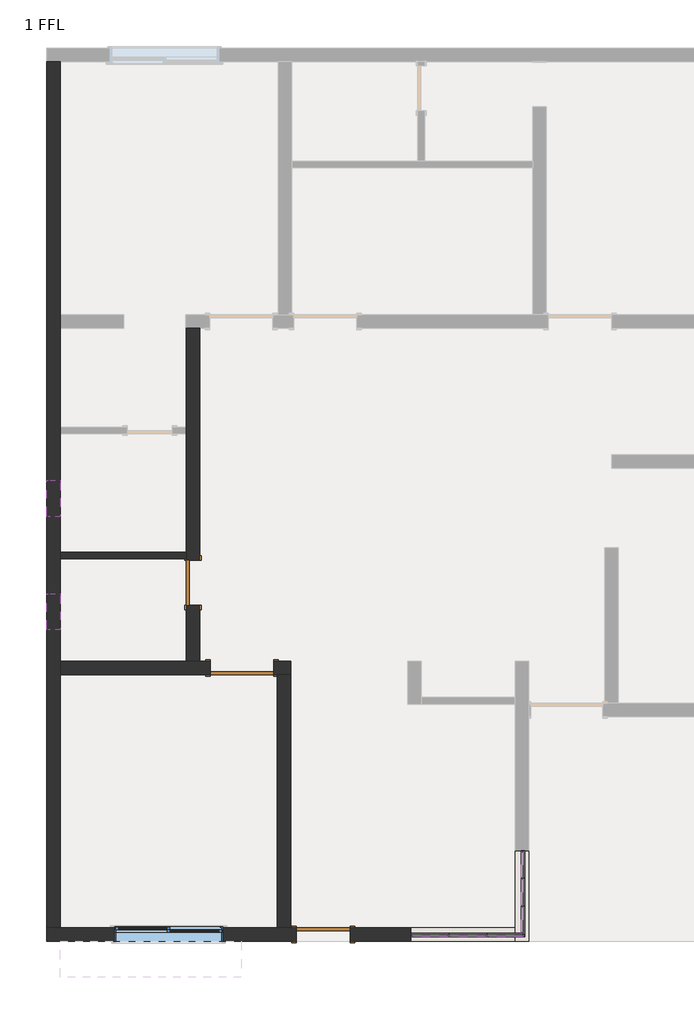
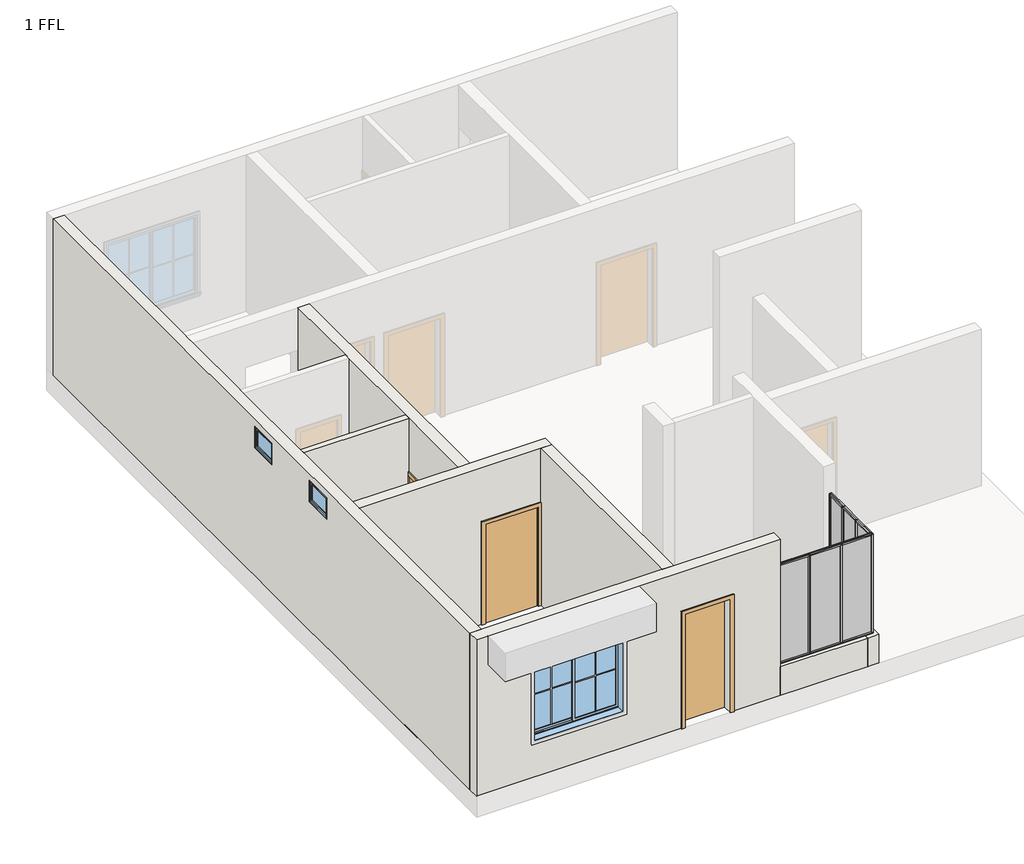
# One storey, part 1 of 2: 23 members, 9 plates, 8 walls, 3 doors, 3 windows.
"""IFC4 building model written with IfcOpenShell, lengths in millimetres."""

from ifc_helpers import new_model, si_unit, origin, origin_with_axes, place, context, project, spatial, polyline, outline, extrude, faceted_brep, transform, mapped, element, save
from components import single_flush_0848dd25, single_flush_bath_bb98abfd, single_flush_md_2_ea82e2eb, member_0e6c94ff, member_b561e846, member_158a8462, member_dd05f1c1, member_cc9ef0d5, member_a5642750, member_968ff67a, member_910a056f, member_3995c9cc, member_c125f493, member_90203b35, system_panel_glazed_d35b251a, system_panel_glazed_6aed1af6, system_panel_glazed_7e3d14c9, fixed_v_1ea75518, window_sliding_double_89c6b595

model = new_model("IFC4")

# Units and contexts
model_context = context("Model", 3, world=origin())
ifc_project = project(units=[si_unit("LENGTHUNIT", "METRE", prefix="MILLI")], contexts=[model_context])

# Site, building, storey
site = spatial("IfcSite", under=ifc_project)
building = spatial("IfcBuilding", under=site)
storey = spatial("IfcBuildingStorey", under=building, Name="1 FFL", Elevation=0.0)

# Doors
placement = place(None, origin())
single_flush_shape = single_flush_0848dd25(model_context)
element("IfcDoor", 1, ObjectType="Single-Flush", at=placement, inside=storey, context=model_context, shape_type="MappedRepresentation", body=[
    mapped(single_flush_shape, transform((-1780.0942549, -3341.3296941, 0.0), x_axis=(1.0, 0.0, 0.0), y_axis=(0.0, 1.0, 0.0), z_axis=(0.0, 0.0, 1.0))),
])
single_flush_bath_shape = single_flush_bath_bb98abfd(model_context)
element("IfcDoor", 2, ObjectType="Single-Flush : BATH", at=placement, inside=storey, context=model_context, shape_type="MappedRepresentation", body=[
    mapped(single_flush_bath_shape, transform((-2605.5942549, -1895.6547785, 0.0), x_axis=(0.0, 1.0, 0.0), y_axis=(-1.0, 0.0, 0.0), z_axis=(0.0, 0.0, 1.0))),
])
single_flush_md_2_shape = single_flush_md_2_ea82e2eb(model_context)
element("IfcDoor", 3, ObjectType="Single-Flush : MD 2", at=placement, inside=storey, context=model_context, shape_type="MappedRepresentation", body=[
    mapped(single_flush_md_2_shape, transform((-408.4942549, -7846.758484, 0.0), x_axis=(-1.0, 0.0, 0.0), y_axis=(0.0, -1.0, 0.0), z_axis=(0.0, 0.0, 1.0))),
])

# Members
member_shape = member_0e6c94ff(model_context)
element("IfcMember", 4, ObjectType="Rectangular Mullion : 1\" Square", at=placement, inside=storey, context=model_context, shape_type="MappedRepresentation", body=[
    mapped(member_shape, transform((2957.0057451, -7811.7296941, 2743.2), x_axis=(0.0, 0.0, 1.0), y_axis=(-1.0, 0.0, 0.0), z_axis=(0.0, -1.0, 0.0))),
])
element("IfcMember", 5, ObjectType="Rectangular Mullion : 1\" Square", at=placement, inside=storey, context=model_context, shape_type="MappedRepresentation", body=[
    mapped(member_shape, transform((2957.0057451, -6884.6296941, 2743.2), x_axis=(0.0, 0.0, 1.0), y_axis=(-1.0, 0.0, 0.0), z_axis=(0.0, -1.0, 0.0))),
])
element("IfcMember", 6, ObjectType="Rectangular Mullion : 1\" Square", at=placement, inside=storey, context=model_context, shape_type="MappedRepresentation", body=[
    mapped(member_shape, transform((2957.0057451, -6452.8296941, 609.6), x_axis=(0.0, 0.0, -1.0), y_axis=(-1.0, 0.0, 0.0), z_axis=(0.0, 1.0, 0.0))),
])
element("IfcMember", 7, ObjectType="Rectangular Mullion : 1\" Square", at=placement, inside=storey, context=model_context, shape_type="MappedRepresentation", body=[
    mapped(member_shape, transform((2957.0057451, -7379.9296941, 609.6), x_axis=(0.0, 0.0, -1.0), y_axis=(-1.0, 0.0, 0.0), z_axis=(0.0, 1.0, 0.0))),
])
member_2_shape = member_b561e846(model_context)
element("IfcMember", 8, ObjectType="Rectangular Mullion : 1\" Square", at=placement, inside=storey, context=model_context, shape_type="MappedRepresentation", body=[
    mapped(member_2_shape, transform((2957.0057451, -7367.2296941, 609.6), x_axis=(0.0, -1.0, 0.0), y_axis=(-1.0, 0.0, 0.0), z_axis=(0.0, 0.0, -1.0))),
])
element("IfcMember", 9, ObjectType="Rectangular Mullion : 1\" Square", at=placement, inside=storey, context=model_context, shape_type="MappedRepresentation", body=[
    mapped(member_2_shape, transform((2957.0057451, -6897.3296941, 609.6), x_axis=(0.0, -1.0, 0.0), y_axis=(-1.0, 0.0, 0.0), z_axis=(0.0, 0.0, -1.0))),
])
member_3_shape = member_158a8462(model_context)
element("IfcMember", 10, ObjectType="Rectangular Mullion : 1\" Square", at=placement, inside=storey, context=model_context, shape_type="MappedRepresentation", body=[
    mapped(member_3_shape, transform((2957.0057451, -6910.0296941, 609.6), x_axis=(0.0, 0.0, -1.0), y_axis=(-1.0, 0.0, 0.0), z_axis=(0.0, 1.0, 0.0))),
])
element("IfcMember", 11, ObjectType="Rectangular Mullion : 1\" Square", at=placement, inside=storey, context=model_context, shape_type="MappedRepresentation", body=[
    mapped(member_3_shape, transform((2957.0057451, -7354.5296941, 2743.2), x_axis=(0.0, 0.0, 1.0), y_axis=(-1.0, 0.0, 0.0), z_axis=(0.0, -1.0, 0.0))),
])
member_4_shape = member_dd05f1c1(model_context)
element("IfcMember", 12, ObjectType="Rectangular Mullion : 1\" Square", at=placement, inside=storey, context=model_context, shape_type="MappedRepresentation", body=[
    mapped(member_4_shape, transform((2957.0057451, -6427.4296941, 2743.2), x_axis=(0.0, 1.0, 0.0), y_axis=(-1.0, 0.0, 0.0), z_axis=(0.0, 0.0, 1.0))),
])
element("IfcMember", 13, ObjectType="Rectangular Mullion : 1\" Square", at=placement, inside=storey, context=model_context, shape_type="MappedRepresentation", body=[
    mapped(member_4_shape, transform((2957.0057451, -7837.1296941, 609.6), x_axis=(0.0, -1.0, 0.0), y_axis=(-1.0, 0.0, 0.0), z_axis=(0.0, 0.0, -1.0))),
])
member_5_shape = member_cc9ef0d5(model_context)
element("IfcMember", 14, ObjectType="Rectangular Mullion : 1\" Square", at=placement, inside=storey, context=model_context, shape_type="MappedRepresentation", body=[
    mapped(member_5_shape, transform((2977.9478614, -7869.7205876, 2743.2), x_axis=(0.0, 0.0, 1.0), y_axis=(0.0, -1.0, 0.0), z_axis=(1.0, 0.0, 0.0))),
])
element("IfcMember", 15, ObjectType="Rectangular Mullion : 1\" Square", at=placement, inside=storey, context=model_context, shape_type="MappedRepresentation", body=[
    mapped(member_5_shape, transform((1703.7145281, -7869.7205876, 2743.2), x_axis=(0.0, 0.0, 1.0), y_axis=(0.0, -1.0, 0.0), z_axis=(1.0, 0.0, 0.0))),
])
member_6_shape = member_a5642750(model_context)
element("IfcMember", 16, ObjectType="Rectangular Mullion : 1\" Square", at=placement, inside=storey, context=model_context, shape_type="MappedRepresentation", body=[
    mapped(member_6_shape, transform((1072.9478614, -7869.7205876, 609.6), x_axis=(0.0, 0.0, -1.0), y_axis=(0.0, -1.0, 0.0), z_axis=(-1.0, 0.0, 0.0))),
])
member_7_shape = member_968ff67a(model_context)
element("IfcMember", 17, ObjectType="Rectangular Mullion : 1\" Square", at=placement, inside=storey, context=model_context, shape_type="MappedRepresentation", body=[
    mapped(member_7_shape, transform((1703.7145281, -7869.7205876, 615.95), x_axis=(0.0, 0.0, 1.0), y_axis=(0.0, -1.0, 0.0), z_axis=(1.0, 0.0, 0.0))),
])
element("IfcMember", 18, ObjectType="Rectangular Mullion : 1\" Square", at=placement, inside=storey, context=model_context, shape_type="MappedRepresentation", body=[
    mapped(member_7_shape, transform((2977.9478614, -7869.7205876, 615.95), x_axis=(0.0, 0.0, 1.0), y_axis=(0.0, -1.0, 0.0), z_axis=(1.0, 0.0, 0.0))),
])
member_8_shape = member_910a056f(model_context)
element("IfcMember", 19, ObjectType="Rectangular Mullion : 1\" Square", at=placement, inside=storey, context=model_context, shape_type="MappedRepresentation", body=[
    mapped(member_8_shape, transform((2347.1811947, -7869.7205876, 615.95), x_axis=(0.0, 0.0, 1.0), y_axis=(0.0, -1.0, 0.0), z_axis=(1.0, 0.0, 0.0))),
])
element("IfcMember", 20, ObjectType="Rectangular Mullion : 1\" Square", at=placement, inside=storey, context=model_context, shape_type="MappedRepresentation", body=[
    mapped(member_6_shape, transform((2359.8811947, -7869.7205876, 609.6), x_axis=(0.0, 0.0, -1.0), y_axis=(0.0, -1.0, 0.0), z_axis=(-1.0, 0.0, 0.0))),
])
element("IfcMember", 21, ObjectType="Rectangular Mullion : 1\" Square", at=placement, inside=storey, context=model_context, shape_type="MappedRepresentation", body=[
    mapped(member_6_shape, transform((1716.4145281, -7869.7205876, 609.6), x_axis=(0.0, 0.0, -1.0), y_axis=(0.0, -1.0, 0.0), z_axis=(-1.0, 0.0, 0.0))),
])
member_9_shape = member_3995c9cc(model_context)
element("IfcMember", 22, ObjectType="Rectangular Mullion : 1\" Square", at=placement, inside=storey, context=model_context, shape_type="MappedRepresentation", body=[
    mapped(member_9_shape, transform((2347.1811947, -7869.7205876, 2743.2), x_axis=(0.0, 0.0, 1.0), y_axis=(0.0, -1.0, 0.0), z_axis=(1.0, 0.0, 0.0))),
])
member_10_shape = member_c125f493(model_context)
element("IfcMember", 23, ObjectType="Rectangular Mullion : 1\" Square", at=placement, inside=storey, context=model_context, shape_type="MappedRepresentation", body=[
    mapped(member_10_shape, transform((2359.8811947, -7869.7205876, 603.25), x_axis=(1.0, 0.0, 0.0), y_axis=(0.0, -1.0, 0.0), z_axis=(0.0, 0.0, -1.0))),
])
element("IfcMember", 24, ObjectType="Rectangular Mullion : 1\" Square", at=placement, inside=storey, context=model_context, shape_type="MappedRepresentation", body=[
    mapped(member_10_shape, transform((1716.4145281, -7869.7205876, 603.25), x_axis=(1.0, 0.0, 0.0), y_axis=(0.0, -1.0, 0.0), z_axis=(0.0, 0.0, -1.0))),
])
member_11_shape = member_90203b35(model_context)
element("IfcMember", 25, ObjectType="Rectangular Mullion : 1\" Square", at=placement, inside=storey, context=model_context, shape_type="MappedRepresentation", body=[
    mapped(member_11_shape, transform((1072.9478614, -7869.7205876, 2743.2), x_axis=(-1.0, 0.0, 0.0), y_axis=(0.0, -1.0, 0.0), z_axis=(0.0, 0.0, 1.0))),
])
element("IfcMember", 26, ObjectType="Rectangular Mullion : 1\" Square", at=placement, inside=storey, context=model_context, shape_type="MappedRepresentation", body=[
    mapped(member_11_shape, transform((3003.3478614, -7869.7205876, 603.25), x_axis=(1.0, 0.0, 0.0), y_axis=(0.0, -1.0, 0.0), z_axis=(0.0, 0.0, -1.0))),
])

# Plates
system_panel_glazed_shape = system_panel_glazed_d35b251a(model_context)
element("IfcPlate", 27, ObjectType="System Panel : Glazed", at=placement, inside=storey, context=model_context, shape_type="MappedRepresentation", body=[
    mapped(system_panel_glazed_shape, transform((2957.0057451, -6662.3796941, 609.6), x_axis=(0.0, -1.0, 0.0), y_axis=(1.0, 0.0, 0.0), z_axis=(0.0, 0.0, 1.0))),
])
element("IfcPlate", 28, ObjectType="System Panel : Glazed", at=placement, inside=storey, context=model_context, shape_type="MappedRepresentation", body=[
    mapped(system_panel_glazed_shape, transform((2957.0057451, -7602.1796941, 609.6), x_axis=(0.0, -1.0, 0.0), y_axis=(1.0, 0.0, 0.0), z_axis=(0.0, 0.0, 1.0))),
])
element("IfcPlate", 29, ObjectType="System Panel : Glazed", at=placement, inside=storey, context=model_context, shape_type="MappedRepresentation", body=[
    mapped(system_panel_glazed_shape, transform((2957.0057451, -7132.2796941, 609.6), x_axis=(0.0, -1.0, 0.0), y_axis=(1.0, 0.0, 0.0), z_axis=(0.0, 0.0, 1.0))),
])
system_panel_glazed_2_shape = system_panel_glazed_6aed1af6(model_context)
element("IfcPlate", 30, ObjectType="System Panel : Glazed", at=placement, inside=storey, context=model_context, shape_type="MappedRepresentation", body=[
    mapped(system_panel_glazed_2_shape, transform((1394.6811947, -7869.7205876, 609.6), x_axis=(1.0, 0.0, 0.0), y_axis=(0.0, 1.0, 0.0), z_axis=(0.0, 0.0, 1.0))),
])
element("IfcPlate", 31, ObjectType="System Panel : Glazed", at=placement, inside=storey, context=model_context, shape_type="MappedRepresentation", body=[
    mapped(system_panel_glazed_2_shape, transform((2681.6145281, -7869.7205876, 609.6), x_axis=(1.0, 0.0, 0.0), y_axis=(0.0, 1.0, 0.0), z_axis=(0.0, 0.0, 1.0))),
])
element("IfcPlate", 32, ObjectType="System Panel : Glazed", at=placement, inside=storey, context=model_context, shape_type="MappedRepresentation", body=[
    mapped(system_panel_glazed_2_shape, transform((2038.1478614, -7869.7205876, 609.6), x_axis=(1.0, 0.0, 0.0), y_axis=(0.0, 1.0, 0.0), z_axis=(0.0, 0.0, 1.0))),
])
system_panel_glazed_3_shape = system_panel_glazed_7e3d14c9(model_context)
element("IfcPlate", 33, ObjectType="System Panel : Glazed", at=placement, inside=storey, context=model_context, shape_type="MappedRepresentation", body=[
    mapped(system_panel_glazed_3_shape, transform((1394.6811947, -7869.7205876, 615.95), x_axis=(1.0, 0.0, 0.0), y_axis=(0.0, 1.0, 0.0), z_axis=(0.0, 0.0, 1.0))),
])
element("IfcPlate", 34, ObjectType="System Panel : Glazed", at=placement, inside=storey, context=model_context, shape_type="MappedRepresentation", body=[
    mapped(system_panel_glazed_3_shape, transform((2038.1478614, -7869.7205876, 615.95), x_axis=(1.0, 0.0, 0.0), y_axis=(0.0, 1.0, 0.0), z_axis=(0.0, 0.0, 1.0))),
])
element("IfcPlate", 35, ObjectType="System Panel : Glazed", at=placement, inside=storey, context=model_context, shape_type="MappedRepresentation", body=[
    mapped(system_panel_glazed_3_shape, transform((2681.6145281, -7869.7205876, 615.95), x_axis=(1.0, 0.0, 0.0), y_axis=(0.0, 1.0, 0.0), z_axis=(0.0, 0.0, 1.0))),
])

# Walls
element("IfcWall", 36, ObjectType="4.5\"", at=placement, inside=storey, context=model_context, shape_type="SweptSolid", body=[
    extrude(outline(polyline([(-2719.8942549, -1495.6047785), (-4855.6350579, -1495.6047785), (-4855.6350579, -1381.3047785), (-2719.8942549, -1381.3047785), (-2719.8942549, -1495.6047785)])), origin_with_axes(), (0.0, 0.0, 1.0), 3352.8),
])
element("IfcWall", 37, ObjectType="9\"", at=placement, inside=storey, context=model_context, shape_type="Brep", body=[
    faceted_brep([(-5084.2350579, -7961.058484, 0.0), (-865.6942549, -7961.058484, 0.0), (-865.6942549, -7961.058484, 2438.4), (48.7057451, -7961.058484, 2438.4), (48.7057451, -7961.058484, 0.0), (1072.9478614, -7961.058484, 0.0), (1072.9478614, -7961.058484, 609.6), (1072.9478614, -7961.058484, 2743.2), (1072.9478614, -7961.058484, 3352.8), (-5084.2350579, -7961.058484, 3352.8), (-5084.2350579, -7961.058484, 2743.2), (-2105.0146564, -7961.058484, 2438.4), (-2105.0146564, -7961.058484, 762.0), (-3933.8146564, -7961.058484, 762.0), (-3933.8146564, -7961.058484, 2438.4), (-865.6942549, -7732.458484, 2438.4), (-865.6942549, -7732.458484, 0.0), (-954.5942549, -7732.458484, 0.0), (-1183.1942549, -7732.458484, 0.0), (-4855.6350579, -7732.458484, 0.0), (-5084.2350579, -7732.458484, 0.0), (-5084.2350579, -7732.458484, 3352.8), (-4855.6350579, -7732.458484, 3352.8), (-1183.1942549, -7732.458484, 3352.8), (-954.5942549, -7732.458484, 3352.8), (1072.9478614, -7732.458484, 3352.8), (1072.9478614, -7732.458484, 2743.2), (1072.9478614, -7732.458484, 609.6), (1072.9478614, -7732.458484, 0.0), (48.7057451, -7732.458484, 0.0), (48.7057451, -7732.458484, 2438.4), (-2105.0146564, -7732.458484, 2438.4), (-3933.8146564, -7732.458484, 2438.4), (-3933.8146564, -7732.458484, 762.0), (-2105.0146564, -7732.458484, 762.0)], [[[0, 1, 2, 3, 4, 5, 6, 7, 8, 9, 10], [11, 12, 13, 14]], [[15, 16, 17, 18, 19, 20, 21, 22, 23, 24, 25, 26, 27, 28, 29, 30], [31, 32, 33, 34]], [[29, 28, 5, 4]], [[20, 19, 18, 17, 16, 1, 0]], [[9, 8, 25, 24, 23, 22, 21]], [[12, 11, 31, 34]], [[13, 12, 34, 33]], [[14, 13, 33, 32]], [[11, 14, 32, 31]], [[2, 1, 16, 15]], [[3, 2, 15, 30]], [[4, 3, 30, 29]], [[5, 28, 27, 26, 25, 8, 7, 6]], [[9, 21, 20, 0, 10]]]),
])
element("IfcWall", 38, ObjectType="9\"", at=placement, inside=storey, context=model_context, shape_type="Brep", body=[
    faceted_brep([(-4855.6350579, -7732.458484, 3352.8), (-4855.6350579, -7732.458484, 0.0), (-4855.6350579, -3455.6296941, 0.0), (-4855.6350579, -3227.0296941, 0.0), (-4855.6350579, -1495.6047785, 0.0), (-4855.6350579, -1381.3047785, 0.0), (-4855.6350579, 618.9452215, 0.0), (-4855.6350579, 733.2452215, 0.0), (-4855.6350579, 2406.3534118, 0.0), (-4855.6350579, 2634.9534118, 0.0), (-4855.6350579, 6907.5703059, 0.0), (-4855.6350579, 6907.5703059, 3352.8), (-4855.6350579, 2634.9534118, 3352.8), (-4855.6350579, 2406.3534118, 3352.8), (-4855.6350579, 733.2452215, 3352.8), (-4855.6350579, 618.9452215, 3352.8), (-4855.6350579, -1381.3047785, 3352.8), (-4855.6350579, -1495.6047785, 3352.8), (-4855.6350579, -3227.0296941, 3352.8), (-4855.6350579, -3455.6296941, 3352.8), (-4855.6350579, -2085.0922363, 3200.4), (-4855.6350579, -2085.0922363, 2743.2), (-4855.6350579, -2694.6922363, 2743.2), (-4855.6350579, -2694.6922363, 3200.4), (-4855.6350579, -168.4547785, 3200.4), (-4855.6350579, -168.4547785, 2743.2), (-4855.6350579, -778.0547785, 2743.2), (-4855.6350579, -778.0547785, 3200.4), (-5084.2350579, -7732.458484, 0.0), (-5084.2350579, -7732.458484, 3352.8), (-5084.2350579, 6907.5703059, 3352.8), (-5084.2350579, 6907.5703059, 0.0), (-5084.2350579, -2085.0922363, 3200.4), (-5084.2350579, -2694.6922363, 3200.4), (-5084.2350579, -2694.6922363, 2743.2), (-5084.2350579, -2085.0922363, 2743.2), (-5084.2350579, -168.4547785, 3200.4), (-5084.2350579, -778.0547785, 3200.4), (-5084.2350579, -778.0547785, 2743.2), (-5084.2350579, -168.4547785, 2743.2)], [[[0, 1, 2, 3, 4, 5, 6, 7, 8, 9, 10, 11, 12, 13, 14, 15, 16, 17, 18, 19], [20, 21, 22, 23], [24, 25, 26, 27]], [[28, 29, 30, 31], [32, 33, 34, 35], [36, 37, 38, 39]], [[10, 9, 8, 7, 6, 5, 4, 3, 2, 1, 28, 31]], [[0, 19, 18, 17, 16, 15, 14, 13, 12, 11, 30, 29]], [[11, 10, 31, 30]], [[21, 20, 32, 35]], [[22, 21, 35, 34]], [[23, 22, 34, 33]], [[20, 23, 33, 32]], [[25, 24, 36, 39]], [[26, 25, 39, 38]], [[27, 26, 38, 37]], [[24, 27, 37, 36]], [[0, 29, 28, 1]]]),
])
element("IfcWall", 39, ObjectType="9\"", at=placement, inside=storey, context=model_context, shape_type="Brep", body=[
    faceted_brep([(-1246.6942549, -3455.6296941, 2133.6), (-1246.6942549, -3455.6296941, 0.0), (-1183.1942549, -3455.6296941, 0.0), (-954.5942549, -3455.6296941, 0.0), (-954.5942549, -3455.6296941, 3352.8), (-1183.1942549, -3455.6296941, 3352.8), (-4855.6350579, -3455.6296941, 3352.8), (-4855.6350579, -3455.6296941, 0.0), (-2313.4942549, -3455.6296941, 0.0), (-2313.4942549, -3455.6296941, 2133.6), (-954.5942549, -3227.0296941, 0.0), (-1246.6942549, -3227.0296941, 0.0), (-1246.6942549, -3227.0296941, 2133.6), (-2313.4942549, -3227.0296941, 2133.6), (-2313.4942549, -3227.0296941, 0.0), (-2491.2942549, -3227.0296941, 0.0), (-2719.8942549, -3227.0296941, 0.0), (-4855.6350579, -3227.0296941, 0.0), (-4855.6350579, -3227.0296941, 3352.8), (-2719.8942549, -3227.0296941, 3352.8), (-2491.2942549, -3227.0296941, 3352.8), (-954.5942549, -3227.0296941, 3352.8)], [[[0, 1, 2, 3, 4, 5, 6, 7, 8, 9]], [[10, 11, 12, 13, 14, 15, 16, 17, 18, 19, 20, 21]], [[8, 7, 17, 16, 15, 14]], [[3, 2, 1, 11, 10]], [[6, 5, 4, 21, 20, 19, 18]], [[7, 6, 18, 17]], [[4, 3, 10, 21]], [[12, 11, 1, 0]], [[13, 12, 0, 9]], [[14, 13, 9, 8]]]),
])
element("IfcWall", 40, ObjectType="9\"", at=placement, inside=storey, context=model_context, shape_type="SweptSolid", body=[
    extrude(outline(polyline([(-954.5942549, -3455.6296941), (-954.5942549, -7732.458484), (-1183.1942549, -7732.458484), (-1183.1942549, -3455.6296941), (-954.5942549, -3455.6296941)])), origin_with_axes(), (0.0, 0.0, 1.0), 3352.8),
])
element("IfcWall", 41, ObjectType="9\"", at=placement, inside=storey, context=model_context, shape_type="Brep", body=[
    faceted_brep([(-2491.2942549, -1514.6547785, 2133.6), (-2491.2942549, -1514.6547785, 0.0), (-2491.2942549, 2406.3534118, 0.0), (-2491.2942549, 2406.3534118, 3352.8), (-2491.2942549, -3227.0296941, 3352.8), (-2491.2942549, -3227.0296941, 0.0), (-2491.2942549, -2276.6547785, 0.0), (-2491.2942549, -2276.6547785, 2133.6), (-2719.8942549, 2406.3534118, 0.0), (-2719.8942549, 733.2452215, 0.0), (-2719.8942549, 618.9452215, 0.0), (-2719.8942549, -1381.3047785, 0.0), (-2719.8942549, -1495.6047785, 0.0), (-2719.8942549, -1514.6547785, 0.0), (-2719.8942549, -1514.6547785, 2133.6), (-2719.8942549, -2276.6547785, 2133.6), (-2719.8942549, -2276.6547785, 0.0), (-2719.8942549, -3227.0296941, 0.0), (-2719.8942549, -3227.0296941, 3352.8), (-2719.8942549, -1495.6047785, 3352.8), (-2719.8942549, -1381.3047785, 3352.8), (-2719.8942549, 618.9452215, 3352.8), (-2719.8942549, 733.2452215, 3352.8), (-2719.8942549, 2406.3534118, 3352.8)], [[[0, 1, 2, 3, 4, 5, 6, 7]], [[8, 9, 10, 11, 12, 13, 14, 15, 16, 17, 18, 19, 20, 21, 22, 23]], [[6, 5, 17, 16]], [[2, 1, 13, 12, 11, 10, 9, 8]], [[4, 3, 23, 22, 21, 20, 19, 18]], [[5, 4, 18, 17]], [[3, 2, 8, 23]], [[14, 13, 1, 0]], [[15, 14, 0, 7]], [[16, 15, 7, 6]]]),
])
element("IfcWall", 42, ObjectType="9\"", at=placement, inside=storey, context=model_context, shape_type="Brep", body=[
    faceted_brep([(2842.7057451, -6427.4296941, 0.0), (2842.7057451, -7732.458484, 0.0), (2842.7057451, -7961.058484, 0.0), (2842.7057451, -7961.058484, 609.6), (2842.7057451, -7732.458484, 609.6), (2842.7057451, -6427.4296941, 609.6), (3071.3057451, -6427.4296941, 0.0), (3071.3057451, -6427.4296941, 609.6), (3071.3057451, -7961.058484, 609.6), (3071.3057451, -7961.058484, 0.0)], [[[0, 1, 2, 3, 4, 5]], [[6, 7, 8, 9]], [[2, 1, 0, 6, 9]], [[5, 4, 3, 8, 7]], [[0, 5, 7, 6]], [[3, 2, 9, 8]]]),
])
element("IfcWall", 43, ObjectType="9\"", at=placement, inside=storey, context=model_context, shape_type="SweptSolid", body=[
    extrude(outline(polyline([(1072.9478614, -7732.458484), (2842.7057451, -7732.458484), (2842.7057451, -7961.058484), (1072.9478614, -7961.058484), (1072.9478614, -7732.458484)])), origin_with_axes(), (0.0, 0.0, 1.0), 609.6),
])

# Windows
fixed_v_shape = fixed_v_1ea75518(model_context)
element("IfcWindow", 44, ObjectType="Fixed : V", at=placement, inside=storey, context=model_context, shape_type="MappedRepresentation", body=[
    mapped(fixed_v_shape, transform((-4969.9350579, -2351.7922363, 1828.8), x_axis=(0.0, 1.0, 0.0), y_axis=(-1.0, 0.0, 0.0), z_axis=(0.0, 0.0, 1.0))),
])
element("IfcWindow", 45, ObjectType="Fixed : V", at=placement, inside=storey, context=model_context, shape_type="MappedRepresentation", body=[
    mapped(fixed_v_shape, transform((-4969.9350579, -435.1547785, 1828.8), x_axis=(0.0, 1.0, 0.0), y_axis=(-1.0, 0.0, 0.0), z_axis=(0.0, 0.0, 1.0))),
])
window_sliding_double_shape = window_sliding_double_89c6b595(model_context)
element("IfcWindow", 46, ObjectType="Window-Sliding-Double", at=placement, inside=storey, context=model_context, shape_type="MappedRepresentation", body=[
    mapped(window_sliding_double_shape, transform((-3019.4146564, -7842.948484, -152.4), x_axis=(1.0, 0.0, 0.0), y_axis=(0.0, 1.0, 0.0), z_axis=(0.0, 0.0, 1.0))),
])

save(model, "model.ifc")

# Revit data of these elements
# Type "Single-Flush"
#   Type Mark = "8"
#   Construction Type Id = "MDOOR"
#   Assembly Code = "C1020"
#   Analytic Construction = "Metal"
#   Thickness = 0' - 2"
#   Heat Transfer Coefficient (U) = 0.651978 BTU/(h·ft²·°F)
#   Height = 7' - 0"
#   Trim Projection Ext = 0' - 1"
#   Trim Projection Int = 0' - 1"
#   Trim Width = 0' - 3"
#   Width = 3' - 6"
#   Define Thermal Properties by = 1
#   Door Material = Door - Panel
#   Frame Material = Door - Frame
#   Visual Light Transmittance = 0
#   Solar Heat Gain Coefficient = 0
#   Function = (empty or 0)
#   Wall Closure = (empty or 0)
# Type "Single-Flush : BATH"
#   Type Mark = "9"
#   Construction Type Id = "MDOOR"
#   Assembly Code = "C1020"
#   Analytic Construction = "Metal"
#   Thickness = 0' - 2"
#   Heat Transfer Coefficient (U) = 0.651978 BTU/(h·ft²·°F)
#   Height = 7' - 0"
#   Trim Projection Ext = 0' - 1"
#   Trim Projection Int = 0' - 1"
#   Trim Width = 0' - 3"
#   Width = 2' - 6"
#   Define Thermal Properties by = 1
#   Door Material = Door - Panel
#   Frame Material = Door - Frame
#   Visual Light Transmittance = 0
#   Solar Heat Gain Coefficient = 0
#   Function = (empty or 0)
#   Wall Closure = (empty or 0)
# Type "Single-Flush : MD 2"
#   Type Mark = "11"
#   Construction Type Id = "MDOOR"
#   Assembly Code = "C1020"
#   Analytic Construction = "Metal"
#   Thickness = 0' - 2"
#   Heat Transfer Coefficient (U) = 0.651978 BTU/(h·ft²·°F)
#   Height = 8' - 0"
#   Trim Projection Ext = 0' - 1"
#   Trim Projection Int = 0' - 1"
#   Trim Width = 0' - 3"
#   Width = 3' - 0"
#   Define Thermal Properties by = 1
#   Door Material = Door - Panel
#   Frame Material = Door - Frame
#   Visual Light Transmittance = 0
#   Solar Heat Gain Coefficient = 0
#   Function = (empty or 0)
#   Wall Closure = (empty or 0)
# Type "Rectangular Mullion : 1\" Square"
#   built-in parameter 1007304 = 0.0833333 (stored number, unit not read)
#   built-in parameter 1007301 = 0.0416667 (stored number, unit not read)
#   built-in parameter 1007300 = 0.0416667 (stored number, unit not read)
# Type "System Panel : Glazed"
#   Construction Type Id = "GSP4R"
#   Analytic Construction = "1/8 in Pilkington single glazing"
#   Visual Light Transmittance = 0.9
#   Solar Heat Gain Coefficient = 0.86
#   Heat Transfer Coefficient (U) = 1.18115 BTU/(h·ft²·°F)
#   Define Thermal Properties by = 1
# Type "4.5\""
#   Assembly Code = "B2010"
#   Layers, outside or top first: 0' - 4 1/2" no material (function 1)
# Type "9\""
#   Assembly Code = "B2010"
#   Layers, outside or top first: 0' - 9" no material (function 1)
# Type "Fixed : V"
#   Type Mark = "20"
#   Construction Type Id = "GSP4R"
#   Assembly Code = "B2020100"
#   Analytic Construction = "1/8 in Pilkington single glazing"
#   Visual Light Transmittance = 0.9
#   Solar Heat Gain Coefficient = 0.78
#   Heat Transfer Coefficient (U) = 0.6496 BTU/(h·ft²·°F)
#   Height = 1' - 6"
#   Default Sill Height = 3' - 0"
#   Width = 2' - 0"
#   Window Inset = 0' - 0 3/4"
#   Define Thermal Properties by = 1
#   Glass Pane Material = Glass
#   Sash Material = Sash
#   Wall Closure = (empty or 0)
# Type "Window-Sliding-Double"
#   Type Mark = "19"
#   Fire Rating = "0.5h"
#   Assembly Code = "B2020100"
#   Analytic Construction = "Double glazing - domestic"
#   Window Inset [instance default] = 0' - 0"
#   Wall Thickness [instance default] = 0' - 6"
#   Visual Light Transmittance = 0.81
#   Thermal Resistance (R) = 1.8146 (h·ft²·°F)/BTU
#   Solar Heat Gain Coefficient = 0.76
#   Muntin Width = 2' - 8 5/8"
#   Muntin Height = 5' - 0 1/4"
#   Interior Wall Closure [instance default] = 0' - 2 3/4"
#   Heat Transfer Coefficient (U) = 0.5511 BTU/(h·ft²·°F)
#   Frame Extension [instance default] = 0' - 0 1/4"
#   Exterior Wall Closure [instance default] = 0' - 1 1/4"
#   Rough Width = 6' - 0 1/2"
#   Rough Height = 5' - 6 1/2"
#   Height = 5' - 6"
#   Extension Jamb [instance default] = 0' - 2 3/4"
#   Default Sill Height = 3' - 0"
#   Width = 6' - 0"
#   Interior Trim Visibility [instance default] = yes
#   Indicator Visibility [instance default] = yes
#   Exterior Trim Visibility [instance default] = yes
#   Muntin Visibility = yes
#   Extension Jamb Visibility [instance default] = yes
#   Muntin Pattern = Muntin Pattern_2x2 : Muntin Pattern_2x2
#   Interior Trim Material = Wood - Stained
#   Interior Trim = Trim-Window-Interior-Flat : Picture Frame
#   Interior Frame Material = Wood - Stained
#   Glass Panel Material = Glass
#   Exterior Trim Material = Clad - White
#   Exterior Trim = Trim-Window-Exterior-Flat : with Sill
#   Exterior Frame Material = Clad - White
#   Wall Closure = (empty or 0)
# Element 1 (IfcDoor, "Single-Flush")
#   Phase Created = New Construction
#   Materials on its faces: "Door - Frame", "Door - Panel"
# Element 2 (IfcDoor, "Single-Flush : BATH")
#   Phase Created = New Construction
#   Materials on its faces: "Door - Frame", "Door - Panel"
# Element 3 (IfcDoor, "Single-Flush : MD 2")
#   Phase Created = New Construction
#   Materials on its faces: "Door - Frame", "Door - Panel"
# Elements 4, 5, 6, 7, 8, 9, 10, 11, 12, 13, 14, 15, 16, 17, 18, 19, 20, 21, 22, 23, 24, 25, 26 (IfcMember, "Rectangular Mullion : 1\" Square")
#   Phase Created = New Construction
#   Materials on its faces: "Aluminum"
# Elements 27, 28, 29, 30, 31, 32, 33, 34, 35 (IfcPlate, "System Panel : Glazed")
#   Phase Created = New Construction
#   Materials on its faces: "Glass"
# Element 36 (IfcWall, "4.5\"")
#   Top Offset = 0' - 0"
#   Base Offset = 0' - 0"
#   wall height = 11' - 0"
#   Phase Created = New Construction
#   Base Constraint = 1 FFL
#   Top Constraint = 2 FIRST FLOOR BASE
#   Materials on its faces: "Default Wall"
# Element 37 (IfcWall, "9\"")
#   Top Offset = 0' - 0"
#   Base Offset = 0' - 0"
#   wall height = 11' - 0"
#   Phase Created = New Construction
#   Base Constraint = 1 FFL
#   Top Constraint = 2 FIRST FLOOR BASE
#   Materials on its faces: "Default Wall", "outer wall"
# Elements 38, 39, 40, 41 (IfcWall, "9\"")
#   Top Offset = 0' - 0"
#   Base Offset = 0' - 0"
#   wall height = 11' - 0"
#   Phase Created = New Construction
#   Base Constraint = 1 FFL
#   Top Constraint = 2 FIRST FLOOR BASE
#   Materials on its faces: "Default Wall"
# Elements 42, 43 (IfcWall, "9\"")
#   Top Offset = 0' - 0"
#   Base Offset = 0' - 0"
#   Unconnected Height = 2' - 0"
#   wall height = 2' - 0"
#   Phase Created = New Construction
#   Base Constraint = 1 FFL
#   Materials on its faces: "Default Wall", "outer wall"
# Element 44 (IfcWindow, "Fixed : V")
#   Mark = "3"
#   Phase Created = New Construction
#   Materials on its faces: "Sash", "Glass"
# Element 45 (IfcWindow, "Fixed : V")
#   Mark = "4"
#   Phase Created = New Construction
#   Materials on its faces: "Sash", "Glass"
# Element 46 (IfcWindow, "Window-Sliding-Double")
#   Mark = "2"
#   Window Inset = 0' - 0"
#   Interior Wall Closure = 0' - 2 3/4"
#   Frame Extension = 0' - 0 1/4"
#   Exterior Wall Closure = 0' - 1 1/4"
#   Interior Trim Visibility = yes
#   Indicator Visibility = yes
#   Exterior Trim Visibility = yes
#   Phase Created = New Construction
#   Materials on its faces: "Wood - Stained", "Glass", "Clad - White"
# Materials
#   "Door - Panel": class "Wood", colour RGB 210 159 95, transparency 0, Cost = 0
#   "Door - Frame": colour RGB 118 70 51, transparency 0, Cost = 0
#   "Glass": class "Glass", colour RGB 0 128 192, transparency 0.75, Description = "Soda Lime Glass", Cost = 0
#   "Sash": class "Wood", colour RGB 224 178 126, transparency 0, Cost = 0
#   "Wood - Stained": class "Wood", colour RGB 224 178 126, transparency 0, Cost = 0
#   "Clad - White": class "Wood", colour RGB 242 242 238, transparency 0, Cost = 0
#   "Aluminum": class "Metal", colour RGB 247 247 247, transparency 0, Description = "Aluminum 6061", Cost = 0
#   "Default Wall": colour RGB 128 128 128, transparency 0, Cost = 0
#   "outer wall": class "Generic", colour RGB 85 88 91, transparency 0, Cost = 0
